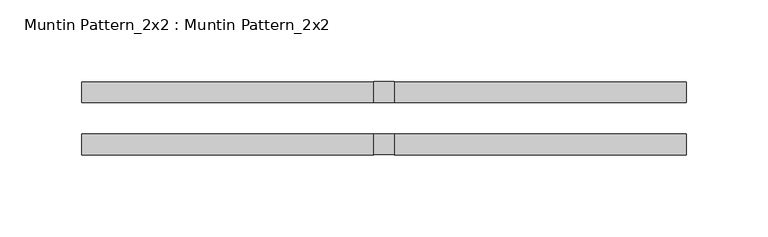
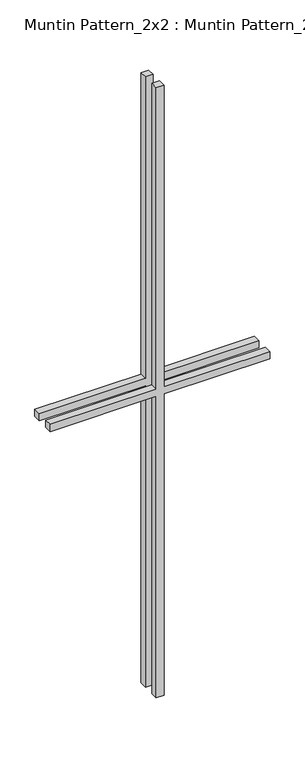
"""IFC4 building model written with IfcOpenShell, lengths in millimetres: proxy geometry, Muntin Pattern_2x2 : Muntin Pattern_2x2."""

from ifc_helpers import new_model, si_unit, frame, origin, place, context, project, spatial, polyline, outline, extrude, source, transform, mapped, element, save


def muntin_pattern_2x2_muntin_pattern_2x2_f03ab90d(model_context):
    return source(origin(), model_context, "Body", "SweptSolid", [
        extrude(outline(polyline([(546.1, -6.35), (546.1, -184.15), (533.4, -184.15), (533.4, -6.35), (0.0, -6.35), (0.0, 6.35), (533.4, 6.35), (533.4, 184.15), (546.1, 184.15), (546.1, 6.35), (1079.5, 6.35), (1079.5, -6.35), (546.1, -6.35)])), frame((0.0, -22.225, 0.0), z_axis=(0.0, 1.0, 0.0), x_axis=(0.0, 0.0, 1.0)), (0.0, 0.0, 1.0), 12.7),
        extrude(outline(polyline([(546.1, -6.35), (546.1, -184.15), (533.4, -184.15), (533.4, -6.35), (0.0, -6.35), (0.0, 6.35), (533.4, 6.35), (533.4, 184.15), (546.1, 184.15), (546.1, 6.35), (1079.5, 6.35), (1079.5, -6.35), (546.1, -6.35)])), frame((0.0, 9.525, 0.0), z_axis=(0.0, 1.0, 0.0), x_axis=(0.0, 0.0, 1.0)), (0.0, 0.0, 1.0), 12.7),
    ])


if __name__ == "__main__":
    model = new_model("IFC4")
    model_context = context("Model", 3, world=origin())
    ifc_project = project(units=[si_unit("LENGTHUNIT", "METRE", prefix="MILLI")], contexts=[model_context])
    site = spatial("IfcSite", under=ifc_project)
    building = spatial("IfcBuilding", under=site)
    placement = place(None, origin())
    muntin_pattern_2x2_muntin_pattern_2x2_shape = muntin_pattern_2x2_muntin_pattern_2x2_f03ab90d(model_context)
    element("IfcBuildingElementProxy", 1, Name="Muntin Pattern_2x2 : Muntin Pattern_2x2", ObjectType="Muntin Pattern_2x2 : Muntin Pattern_2x2", at=placement, inside=building, context=model_context, shape_type="MappedRepresentation", body=[
        mapped(muntin_pattern_2x2_muntin_pattern_2x2_shape, transform((0.0, 0.0, 0.0), x_axis=(1.0, 0.0, 0.0), y_axis=(0.0, 1.0, 0.0), z_axis=(0.0, 0.0, 1.0))),
    ])
    save(model, "model.ifc")

# Revit data of these elements
# Type "Muntin Pattern_2x2 : Muntin Pattern_2x2"
#   Width [instance default] = 4' - 0"
#   Thickness = 0' - 0 1/2"
#   Height [instance default] = 4' - 0"
#   Distance = 0' - 0 3/4"
#   Interior Material [instance default] = none
#   Exterior Material [instance default] = none
#   Default Elevation = 0
# Element 1 (IfcBuildingElementProxy, "Muntin Pattern_2x2 : Muntin Pattern_2x2")
#   Width = 1' - 2 1/2"
#   Height = 3' - 6 1/2"
#   Interior Material = Wood - Stained
#   Exterior Material = Clad - White
#   Materials on its faces: "Clad - White", "Wood - Stained"
# Materials
#   "Clad - White": class "Wood", colour RGB 242 242 238, transparency 0, Cost = 0
#   "Wood - Stained": class "Wood", colour RGB 224 178 126, transparency 0, Cost = 0
